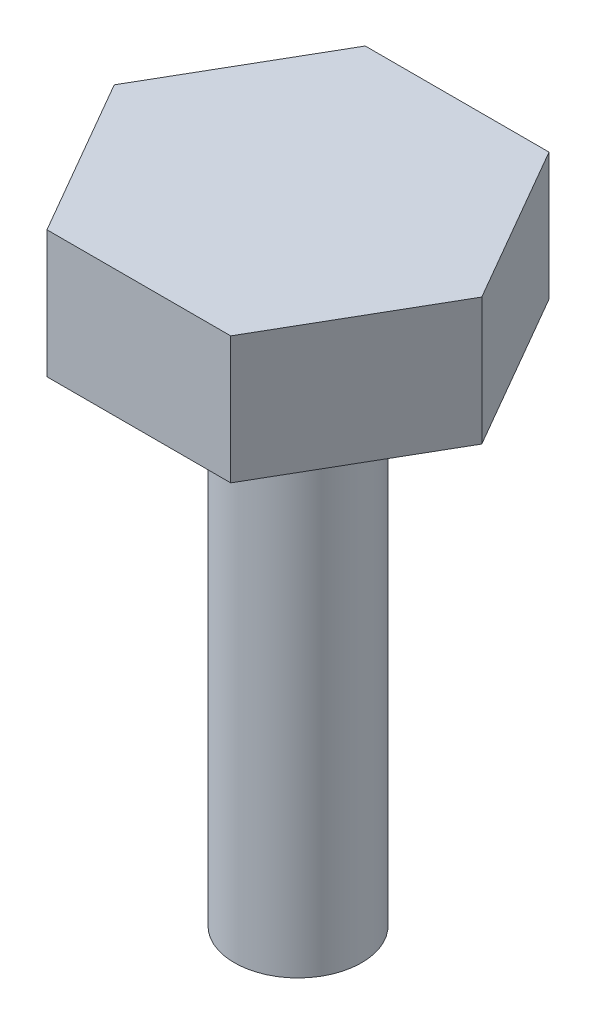
from build123d import *

# Parameters (mm, degrees)
HEX_HEAD_50AF_X20_DEPTH = 20
SHANK_SKETCH_20_R       = 10
SHANK_20X80_DEPTH       = 80


with BuildPart() as part:
    # Hex Head Sketch 50AF → Hex Head 50AF x20 (new body)
    with BuildSketch(Plane(origin=(0, 0, 0), x_dir=(1, 0, 0), z_dir=(0, 1, 0))):
        Polygon((28.867513459, 0), (14.43375673, 25), (-14.43375673, 25), (-28.867513459, 0), (-14.43375673, -25), (14.43375673, -25), align=None)
    extrude(amount=HEX_HEAD_50AF_X20_DEPTH)

    # Shank Sketch Ø20 → Shank Ø20x80 (add)
    with BuildSketch(Plane.XZ):
        with Locations(Location((0, 0, 0), (0, 0, 270))):
            Circle(SHANK_SKETCH_20_R)
    extrude(amount=SHANK_20X80_DEPTH)


solid = part.part
